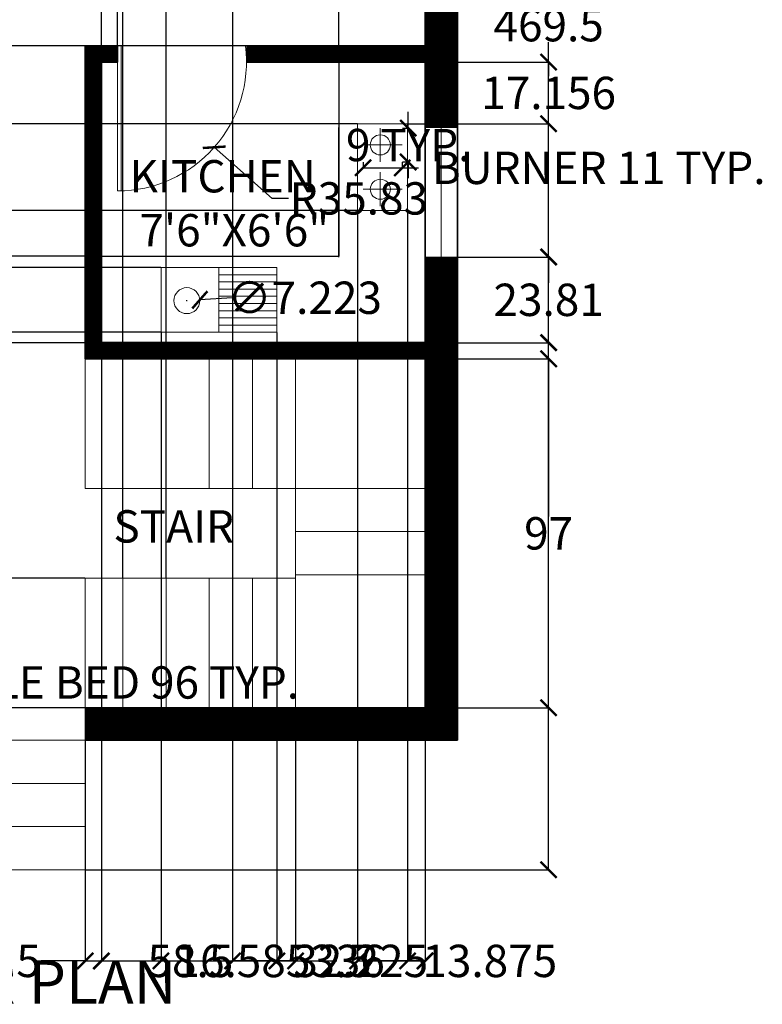
# Model space of a CAD drawing. Units: inches. Extents: x -1 to 426, y -6 to 532.
# Tile 2 of 4: x 219 to 426, y -6 to 267. Entities that reach past the tile are written whole.
import ezdxf

# ---------------------------------------------------------------- set-up
doc = ezdxf.new("R2010")
doc.units = ezdxf.units.IN
doc.header["$MEASUREMENT"] = 0
for name, color, linetype, lineweight in [('A-ANNO-DIMS', 2, 'Continuous', 18), ('A-ANNO-TEXT', 7, 'Continuous', 35), ('A-AREA-IDEN', 7, 'Continuous', 25), ('A-DOOR', 3, 'Continuous', 18), ('A-EQPM', 8, 'Continuous', 18), ('A-FLOR-CASE', 8, 'Continuous', 25), ('A-FLOR-FIXT', 8, 'Continuous', 18), ('A-FLOR-STRS', 42, 'Continuous', 18), ('A-GLAZ', 4, 'Continuous', 18)]:
    doc.layers.add(name, color=color, linetype=linetype, lineweight=lineweight)
doc.layers.add('A-WALL', color=159, linetype='Continuous', lineweight=35, true_color=0x223569)
doc.layers.add('A-WALL-PATT', color=177, linetype='Continuous', lineweight=13, true_color=0x2c4178)
doc.styles.get("Standard").update_dxf_attribs({"font": 'arial.ttf'})
doc.dimstyles.get("Standard").update_dxf_attribs({"dimtxt": 9, "dimasz": 4.5, "dimexe": 0.18, "dimexo": 0.0625, "dimgap": 0.09, "dimtad": 0, "dimtih": 1, "dimtoh": 1, "dimdec": 1, "dimzin": 0, "dimdsep": 46, "dimlunit": 4, "dimtxsty": 'Standard', "dimblk": 'ARCHTICK', "dimcen": 0.09, "dimadec": 0, "dimazin": 0, "dimtfac": 1, "dimtdec": 1, "dimtofl": 0, "dimtmove": 0, "dimatfit": 3, "dimfxl": 1, "dimtolj": 1, "dimtzin": 0, "dimarcsym": 0})

# ---------------------------------------------------------------- blocks, each defined once
blk = doc.blocks.new('WIN-36IN')
for p, q in [((0, 4.5), (36, 4.5)), ((0, -4.5), (0, 4.5)), ((36, 4.5), (36, -4.5)), ((0, 0), (36, 0)), ((36, -4.5), (0, -4.5))]:
    blk.add_line(p, q)
blk = doc.blocks.new('COOKTOP-BURNER')
for q in [(0, 4.66), (-4.8, 0), (6.12, 0), (0, -4.75)]:
    blk.add_line((0, 0), q)
blk.add_circle((0, 0), 2.79)
blk = doc.blocks.new('_ArchTick')
at = {"color": 0, "linetype": 'ByBlock', "const_width": 0.15}
blk.add_lwpolyline([(-0.5, -0.5), (0.5, 0.5)], dxfattribs=at)
blk = doc.blocks.new('*D11')
at = {"layer": 'A-ANNO-DIMS', "color": 0, "lineweight": -2, "transparency": 16777216}
for p, q in [((72.72, 97.36), (72.72, 82.85)), ((168.72, 97.36), (168.72, 82.85)), ((72.72, 83.03), (168.72, 83.03)), ((168.72, 83.03), (173.22, 83.03))]:
    blk.add_line(p, q, dxfattribs=at)
at = {"layer": 'Defpoints', "color": 0, "transparency": 16777216}
for p in [(72.72, 97.43), (168.72, 97.43), (168.72, 83.03)]:
    blk.add_point(p, dxfattribs=at)
at = {"layer": 'A-ANNO-DIMS', "color": 0, "lineweight": -2, "transparency": 16777216, "xscale": 4.5, "yscale": 4.5, "zscale": 4.5, "rotation": 180}
blk.add_blockref('_ArchTick', (72.72, 83.03), dxfattribs=at)
at = {"layer": 'A-ANNO-DIMS', "color": 0, "lineweight": -2, "transparency": 16777216, "xscale": 4.5, "yscale": 4.5, "zscale": 4.5}
blk.add_blockref('_ArchTick', (168.72, 83.03), dxfattribs=at)
at = {"layer": 'A-ANNO-DIMS', "color": 0, "transparency": 16777216, "insert": (237.26, 83.03), "char_height": 9, "attachment_point": 5}
blk.add_mtext('\\A1;DOUBLE BED 96 TYP.', dxfattribs=at)
blk = doc.blocks.new('*D15')
at = {"layer": 'A-ANNO-DIMS', "color": 0, "lineweight": -2, "transparency": 16777216}
for p, q in [((314.58, 227.64), (314.58, 225.89)), ((325.49, 227.64), (325.49, 225.89)), ((314.58, 226.07), (325.49, 226.07)), ((325.49, 226.07), (329.99, 226.07))]:
    blk.add_line(p, q, dxfattribs=at)
at = {"layer": 'Defpoints', "color": 0, "transparency": 16777216}
for p in [(314.58, 227.71), (325.49, 227.71), (325.49, 226.07)]:
    blk.add_point(p, dxfattribs=at)
at = {"layer": 'A-ANNO-DIMS', "color": 0, "lineweight": -2, "transparency": 16777216, "xscale": 4.5, "yscale": 4.5, "zscale": 4.5, "rotation": 180}
blk.add_blockref('_ArchTick', (314.58, 226.07), dxfattribs=at)
at = {"layer": 'A-ANNO-DIMS', "color": 0, "lineweight": -2, "transparency": 16777216, "xscale": 4.5, "yscale": 4.5, "zscale": 4.5}
blk.add_blockref('_ArchTick', (325.49, 226.07), dxfattribs=at)
at = {"layer": 'A-ANNO-DIMS', "color": 0, "transparency": 16777216, "insert": (380.08, 226.07), "char_height": 9, "attachment_point": 5}
blk.add_mtext('\\A1;BURNER 11 TYP.', dxfattribs=at)
blk = doc.blocks.new('*D16')
at = {"layer": 'A-ANNO-DIMS', "color": 0, "lineweight": -2, "transparency": 16777216}
for p, q in [((327.13, 237.11), (327.13, 241.61)), ((325.55, 237.11), (327.31, 237.11)), ((325.55, 227.71), (327.31, 227.71)), ((327.13, 227.71), (327.13, 223.21))]:
    blk.add_line(p, q, dxfattribs=at)
at = {"layer": 'Defpoints', "color": 0, "transparency": 16777216}
for p in [(325.49, 237.11), (327.13, 237.11), (325.49, 227.71)]:
    blk.add_point(p, dxfattribs=at)
at = {"layer": 'A-ANNO-DIMS', "color": 0, "lineweight": -2, "transparency": 16777216, "xscale": 4.5, "yscale": 4.5, "zscale": 4.5}
for p, rotation in [((327.13, 237.11), 270), ((327.13, 227.71), 90)]:
    blk.add_blockref('_ArchTick', p, dxfattribs=dict(at, rotation=rotation))
at = {"layer": 'A-ANNO-DIMS', "color": 0, "transparency": 16777216, "insert": (327.13, 232.41), "char_height": 9, "attachment_point": 5}
blk.add_mtext('\\A1;9 TYP.', dxfattribs=at)
blk = doc.blocks.new('*D18')
at = {"layer": 'A-ANNO-DIMS', "color": 0, "lineweight": -2, "transparency": 16777216}
for p, q in [((340.89, 500.48), (366.36, 500.48)), ((366.18, 500.48), (366.18, 270.42)), ((366.18, 30.98), (366.18, 261.05)), ((237.39, 30.98), (366.36, 30.98))]:
    blk.add_line(p, q, dxfattribs=at)
at = {"layer": 'Defpoints', "color": 0, "transparency": 16777216}
for p in [(340.82, 500.48), (366.18, 500.48), (237.32, 30.98)]:
    blk.add_point(p, dxfattribs=at)
at = {"layer": 'A-ANNO-DIMS', "color": 0, "lineweight": -2, "transparency": 16777216, "xscale": 4.5, "yscale": 4.5, "zscale": 4.5}
for p, rotation in [((366.18, 500.48), 90), ((366.18, 30.98), 270)]:
    blk.add_blockref('_ArchTick', p, dxfattribs=dict(at, rotation=rotation))
at = {"layer": 'A-ANNO-DIMS', "color": 0, "transparency": 16777216, "insert": (366.18, 265.73), "char_height": 9, "attachment_point": 5}
blk.add_mtext('\\A1;469.5', dxfattribs=at)
blk = doc.blocks.new('*D21')
at = {"layer": 'A-ANNO-DIMS', "color": 0, "lineweight": -2, "transparency": 16777216}
for p, q in [((188.82, 30.92), (188.82, 5.45)), ((237.32, 30.92), (237.32, 5.45)), ((188.82, 5.63), (201.08, 5.63)), ((237.32, 5.63), (225.07, 5.63))]:
    blk.add_line(p, q, dxfattribs=at)
at = {"layer": 'Defpoints', "color": 0, "transparency": 16777216}
for p in [(188.82, 30.98), (237.32, 30.98), (237.32, 5.63)]:
    blk.add_point(p, dxfattribs=at)
at = {"layer": 'A-ANNO-DIMS', "color": 0, "lineweight": -2, "transparency": 16777216, "xscale": 4.5, "yscale": 4.5, "zscale": 4.5, "rotation": 180}
blk.add_blockref('_ArchTick', (188.82, 5.63), dxfattribs=at)
at = {"layer": 'A-ANNO-DIMS', "color": 0, "lineweight": -2, "transparency": 16777216, "xscale": 4.5, "yscale": 4.5, "zscale": 4.5}
blk.add_blockref('_ArchTick', (237.32, 5.63), dxfattribs=at)
at = {"layer": 'A-ANNO-DIMS', "color": 0, "transparency": 16777216, "insert": (213.07, 5.63), "char_height": 9, "attachment_point": 5}
blk.add_mtext('\\A1;48.5', dxfattribs=at)
blk = doc.blocks.new('*D23')
at = {"layer": 'A-ANNO-DIMS', "color": 0, "lineweight": -2, "transparency": 16777216}
for p, q in [((278.32, 491.42), (278.32, 5.45)), ((331.82, 491.42), (331.82, 5.45)), ((278.32, 5.63), (293.26, 5.63)), ((331.82, 5.63), (316.89, 5.63))]:
    blk.add_line(p, q, dxfattribs=at)
at = {"layer": 'Defpoints', "color": 0, "transparency": 16777216}
for p in [(278.32, 491.48), (331.82, 491.48), (331.82, 5.63)]:
    blk.add_point(p, dxfattribs=at)
at = {"layer": 'A-ANNO-DIMS', "color": 0, "lineweight": -2, "transparency": 16777216, "xscale": 4.5, "yscale": 4.5, "zscale": 4.5, "rotation": 180}
blk.add_blockref('_ArchTick', (278.32, 5.63), dxfattribs=at)
at = {"layer": 'A-ANNO-DIMS', "color": 0, "lineweight": -2, "transparency": 16777216, "xscale": 4.5, "yscale": 4.5, "zscale": 4.5}
blk.add_blockref('_ArchTick', (331.82, 5.63), dxfattribs=at)
at = {"layer": 'A-ANNO-DIMS', "color": 0, "transparency": 16777216, "insert": (305.07, 5.63), "char_height": 9, "attachment_point": 5}
blk.add_mtext('\\A1;53.5', dxfattribs=at)
blk = doc.blocks.new('*D31')
at = {"layer": 'A-ANNO-DIMS', "color": 0, "lineweight": -2, "transparency": 16777216}
for p, q in [((331.89, 201.29), (366.36, 201.29)), ((366.18, 201.29), (366.18, 194.08)), ((366.18, 177.48), (366.18, 184.7)), ((331.89, 177.48), (366.36, 177.48))]:
    blk.add_line(p, q, dxfattribs=at)
at = {"layer": 'Defpoints', "color": 0, "transparency": 16777216}
for p in [(331.82, 201.29), (366.18, 201.29), (331.82, 177.48)]:
    blk.add_point(p, dxfattribs=at)
at = {"layer": 'A-ANNO-DIMS', "color": 0, "lineweight": -2, "transparency": 16777216, "xscale": 4.5, "yscale": 4.5, "zscale": 4.5}
for p, rotation in [((366.18, 201.29), 90), ((366.18, 177.48), 270)]:
    blk.add_blockref('_ArchTick', p, dxfattribs=dict(at, rotation=rotation))
at = {"layer": 'A-ANNO-DIMS', "color": 0, "transparency": 16777216, "insert": (366.18, 189.39), "char_height": 9, "attachment_point": 5}
blk.add_mtext('\\A1;23.81', dxfattribs=at)
blk = doc.blocks.new('*D32')
at = {"layer": 'A-ANNO-DIMS', "color": 0, "lineweight": -2, "transparency": 16777216}
for p, q in [((331.76, 293.06), (17.79, 293.06)), ((17.97, 293.06), (17.97, 281.21)), ((17.97, 259.98), (17.97, 271.83)), ((331.76, 259.98), (17.79, 259.98))]:
    blk.add_line(p, q, dxfattribs=at)
at = {"layer": 'Defpoints', "color": 0, "transparency": 16777216}
for p in [(17.97, 293.06), (331.82, 293.06), (331.82, 259.98)]:
    blk.add_point(p, dxfattribs=at)
at = {"layer": 'A-ANNO-DIMS', "color": 0, "lineweight": -2, "transparency": 16777216, "xscale": 4.5, "yscale": 4.5, "zscale": 4.5}
for p, rotation in [((17.97, 293.06), 90), ((17.97, 259.98), 270)]:
    blk.add_blockref('_ArchTick', p, dxfattribs=dict(at, rotation=rotation))
at = {"layer": 'A-ANNO-DIMS', "color": 0, "transparency": 16777216, "insert": (17.97, 276.52), "char_height": 9, "attachment_point": 5}
blk.add_mtext('\\A1;33.08', dxfattribs=at)
blk = doc.blocks.new('*D34')
at = {"layer": 'A-ANNO-DIMS', "color": 0, "lineweight": -2, "transparency": 16777216}
for p, q in [((237.26, 111.98), (17.79, 111.98)), ((17.97, 111.98), (17.97, 98.67)), ((17.97, 75.98), (17.97, 89.29)), ((237.26, 75.98), (17.79, 75.98))]:
    blk.add_line(p, q, dxfattribs=at)
at = {"layer": 'Defpoints', "color": 0, "transparency": 16777216}
for p in [(17.97, 111.98), (237.32, 111.98), (237.32, 75.98)]:
    blk.add_point(p, dxfattribs=at)
at = {"layer": 'A-ANNO-DIMS', "color": 0, "lineweight": -2, "transparency": 16777216, "xscale": 4.5, "yscale": 4.5, "zscale": 4.5}
for p, rotation in [((17.97, 111.98), 90), ((17.97, 75.98), 270)]:
    blk.add_blockref('_ArchTick', p, dxfattribs=dict(at, rotation=rotation))
at = {"layer": 'A-ANNO-DIMS', "color": 0, "transparency": 16777216, "insert": (17.97, 93.98), "char_height": 9, "attachment_point": 5}
blk.add_mtext('\\A1;36', dxfattribs=at)
blk = doc.blocks.new('*D35')
at = {"layer": 'A-ANNO-DIMS', "color": 0, "lineweight": -2, "transparency": 16777216}
for p, q in [((247.82, 112.04), (247.82, 526.02)), ((247.82, 525.84), (259.82, 525.84)), ((259.82, 112.04), (259.82, 526.02)), ((259.82, 525.84), (264.32, 525.84))]:
    blk.add_line(p, q, dxfattribs=at)
at = {"layer": 'Defpoints', "color": 0, "transparency": 16777216}
for p in [(259.82, 525.84), (247.82, 111.98), (259.82, 111.98)]:
    blk.add_point(p, dxfattribs=at)
at = {"layer": 'A-ANNO-DIMS', "color": 0, "lineweight": -2, "transparency": 16777216, "xscale": 4.5, "yscale": 4.5, "zscale": 4.5, "rotation": 180}
blk.add_blockref('_ArchTick', (247.82, 525.84), dxfattribs=at)
at = {"layer": 'A-ANNO-DIMS', "color": 0, "lineweight": -2, "transparency": 16777216, "xscale": 4.5, "yscale": 4.5, "zscale": 4.5}
blk.add_blockref('_ArchTick', (259.82, 525.84), dxfattribs=at)
at = {"layer": 'A-ANNO-DIMS', "color": 0, "transparency": 16777216, "insert": (270.39, 525.84), "char_height": 9, "attachment_point": 5}
blk.add_mtext('\\A1;12', dxfattribs=at)
blk = doc.blocks.new('*D36')
at = {"layer": 'A-ANNO-DIMS', "color": 0, "lineweight": -2, "transparency": 16777216}
for p, q in [((258.4, 180.34), (258.4, 5.45)), ((290.63, 180.34), (290.63, 5.45)), ((258.4, 5.63), (290.63, 5.63)), ((290.63, 5.63), (295.13, 5.63))]:
    blk.add_line(p, q, dxfattribs=at)
at = {"layer": 'Defpoints', "color": 0, "transparency": 16777216}
for p in [(258.4, 180.4), (290.63, 180.4), (290.63, 5.63)]:
    blk.add_point(p, dxfattribs=at)
at = {"layer": 'A-ANNO-DIMS', "color": 0, "lineweight": -2, "transparency": 16777216, "xscale": 4.5, "yscale": 4.5, "zscale": 4.5, "rotation": 180}
blk.add_blockref('_ArchTick', (258.4, 5.63), dxfattribs=at)
at = {"layer": 'A-ANNO-DIMS', "color": 0, "lineweight": -2, "transparency": 16777216, "xscale": 4.5, "yscale": 4.5, "zscale": 4.5}
blk.add_blockref('_ArchTick', (290.63, 5.63), dxfattribs=at)
at = {"layer": 'A-ANNO-DIMS', "color": 0, "transparency": 16777216, "insert": (313.93, 5.63), "char_height": 9, "attachment_point": 5}
blk.add_mtext('\\A1;32.225', dxfattribs=at)
blk = doc.blocks.new('*D37')
at = {"layer": 'A-ANNO-DIMS', "color": 0, "lineweight": -2, "transparency": 16777216}
for p, q in [((258.34, 198.36), (17.79, 198.36)), ((17.97, 198.36), (17.97, 194.07)), ((17.97, 180.4), (17.97, 184.7)), ((258.34, 180.4), (17.79, 180.4))]:
    blk.add_line(p, q, dxfattribs=at)
at = {"layer": 'Defpoints', "color": 0, "transparency": 16777216}
for p in [(17.97, 198.36), (258.4, 198.36), (258.4, 180.4)]:
    blk.add_point(p, dxfattribs=at)
at = {"layer": 'A-ANNO-DIMS', "color": 0, "lineweight": -2, "transparency": 16777216, "xscale": 4.5, "yscale": 4.5, "zscale": 4.5}
for p, rotation in [((17.97, 198.36), 90), ((17.97, 180.4), 270)]:
    blk.add_blockref('_ArchTick', p, dxfattribs=dict(at, rotation=rotation))
at = {"layer": 'A-ANNO-DIMS', "color": 0, "transparency": 16777216, "insert": (17.97, 189.38), "char_height": 9, "attachment_point": 5}
blk.add_mtext('\\A1;17.96', dxfattribs=at)
blk = doc.blocks.new('*D38')
at = {"layer": 'A-ANNO-DIMS', "color": 0, "lineweight": -2, "transparency": 16777216}
for p, q in [((307.82, 255.54), (307.82, 526.02)), ((307.82, 525.84), (313.23, 525.84)), ((331.82, 525.84), (326.42, 525.84)), ((331.82, 255.54), (331.82, 526.02))]:
    blk.add_line(p, q, dxfattribs=at)
at = {"layer": 'Defpoints', "color": 0, "transparency": 16777216}
for p in [(331.82, 525.84), (307.82, 255.48), (331.82, 255.48)]:
    blk.add_point(p, dxfattribs=at)
at = {"layer": 'A-ANNO-DIMS', "color": 0, "lineweight": -2, "transparency": 16777216, "xscale": 4.5, "yscale": 4.5, "zscale": 4.5, "rotation": 180}
blk.add_blockref('_ArchTick', (307.82, 525.84), dxfattribs=at)
at = {"layer": 'A-ANNO-DIMS', "color": 0, "lineweight": -2, "transparency": 16777216, "xscale": 4.5, "yscale": 4.5, "zscale": 4.5}
blk.add_blockref('_ArchTick', (331.82, 525.84), dxfattribs=at)
at = {"layer": 'A-ANNO-DIMS', "color": 0, "transparency": 16777216, "insert": (319.82, 525.84), "char_height": 9, "attachment_point": 5}
blk.add_mtext('\\A1;24', dxfattribs=at)
blk = doc.blocks.new('*D42')
at = {"layer": 'A-ANNO-DIMS', "color": 0, "lineweight": -2, "transparency": 16777216}
for p, q in [((331.89, 172.98), (366.36, 172.98)), ((366.18, 172.98), (366.18, 129.17)), ((366.18, 75.98), (366.18, 119.8)), ((331.89, 75.98), (366.36, 75.98))]:
    blk.add_line(p, q, dxfattribs=at)
at = {"layer": 'Defpoints', "color": 0, "transparency": 16777216}
for p in [(331.82, 172.98), (366.18, 172.98), (331.82, 75.98)]:
    blk.add_point(p, dxfattribs=at)
at = {"layer": 'A-ANNO-DIMS', "color": 0, "lineweight": -2, "transparency": 16777216, "xscale": 4.5, "yscale": 4.5, "zscale": 4.5}
for p, rotation in [((366.18, 172.98), 90), ((366.18, 75.98), 270)]:
    blk.add_blockref('_ArchTick', p, dxfattribs=dict(at, rotation=rotation))
at = {"layer": 'A-ANNO-DIMS', "color": 0, "transparency": 16777216, "insert": (366.18, 124.48), "char_height": 9, "attachment_point": 5}
blk.add_mtext('\\A1;97', dxfattribs=at)
blk = doc.blocks.new('*D43')
at = {"layer": 'A-ANNO-DIMS', "color": 0, "lineweight": -2, "transparency": 16777216}
for p, q in [((295.82, 75.92), (295.82, 5.45)), ((331.82, 75.92), (331.82, 5.45)), ((295.82, 5.63), (307.29, 5.63)), ((331.82, 5.63), (320.35, 5.63))]:
    blk.add_line(p, q, dxfattribs=at)
at = {"layer": 'Defpoints', "color": 0, "transparency": 16777216}
for p in [(295.82, 75.98), (331.82, 75.98), (331.82, 5.63)]:
    blk.add_point(p, dxfattribs=at)
at = {"layer": 'A-ANNO-DIMS', "color": 0, "lineweight": -2, "transparency": 16777216, "xscale": 4.5, "yscale": 4.5, "zscale": 4.5, "rotation": 180}
blk.add_blockref('_ArchTick', (295.82, 5.63), dxfattribs=at)
at = {"layer": 'A-ANNO-DIMS', "color": 0, "lineweight": -2, "transparency": 16777216, "xscale": 4.5, "yscale": 4.5, "zscale": 4.5}
blk.add_blockref('_ArchTick', (331.82, 5.63), dxfattribs=at)
at = {"layer": 'A-ANNO-DIMS', "color": 0, "transparency": 16777216, "insert": (313.82, 5.63), "char_height": 9, "attachment_point": 5}
blk.add_mtext('\\A1;36', dxfattribs=at)
blk = doc.blocks.new('*D44')
at = {"layer": 'A-ANNO-DIMS', "color": 0, "lineweight": -2, "transparency": 16777216}
for p, q in [((237.32, 75.92), (237.32, 5.45)), ((295.82, 75.92), (295.82, 5.45)), ((237.32, 5.63), (254.76, 5.63)), ((295.82, 5.63), (278.39, 5.63))]:
    blk.add_line(p, q, dxfattribs=at)
at = {"layer": 'Defpoints', "color": 0, "transparency": 16777216}
for p in [(237.32, 75.98), (295.82, 75.98), (295.82, 5.63)]:
    blk.add_point(p, dxfattribs=at)
at = {"layer": 'A-ANNO-DIMS', "color": 0, "lineweight": -2, "transparency": 16777216, "xscale": 4.5, "yscale": 4.5, "zscale": 4.5, "rotation": 180}
blk.add_blockref('_ArchTick', (237.32, 5.63), dxfattribs=at)
at = {"layer": 'A-ANNO-DIMS', "color": 0, "lineweight": -2, "transparency": 16777216, "xscale": 4.5, "yscale": 4.5, "zscale": 4.5}
blk.add_blockref('_ArchTick', (295.82, 5.63), dxfattribs=at)
at = {"layer": 'A-ANNO-DIMS', "color": 0, "transparency": 16777216, "insert": (266.57, 5.63), "char_height": 9, "attachment_point": 5}
blk.add_mtext('\\A1;58.5', dxfattribs=at)
blk = doc.blocks.new('*D45')
at = {"layer": 'A-ANNO-DIMS', "color": 0, "lineweight": -2, "transparency": 16777216}
for p, q in [((241.76, 201.48), (17.79, 201.48)), ((17.97, 201.48), (17.97, 194.09)), ((17.97, 177.48), (17.97, 184.87)), ((241.76, 177.48), (17.79, 177.48))]:
    blk.add_line(p, q, dxfattribs=at)
at = {"layer": 'Defpoints', "color": 0, "transparency": 16777216}
for p in [(17.97, 201.48), (241.82, 201.48), (241.82, 177.48)]:
    blk.add_point(p, dxfattribs=at)
at = {"layer": 'A-ANNO-DIMS', "color": 0, "lineweight": -2, "transparency": 16777216, "xscale": 4.5, "yscale": 4.5, "zscale": 4.5}
for p, rotation in [((17.97, 201.48), 90), ((17.97, 177.48), 270)]:
    blk.add_blockref('_ArchTick', p, dxfattribs=dict(at, rotation=rotation))
at = {"layer": 'A-ANNO-DIMS', "color": 0, "transparency": 16777216, "insert": (17.97, 189.48), "char_height": 9, "attachment_point": 5}
blk.add_mtext('\\A1;24', dxfattribs=at)
blk = doc.blocks.new('*D46')
at = {"layer": 'A-ANNO-DIMS', "color": 0, "lineweight": -2, "transparency": 16777216}
for p, q in [((241.82, 255.54), (241.82, 526.02)), ((241.82, 525.84), (246.32, 525.84)), ((246.32, 255.54), (246.32, 526.02)), ((246.32, 525.84), (250.82, 525.84))]:
    blk.add_line(p, q, dxfattribs=at)
at = {"layer": 'Defpoints', "color": 0, "transparency": 16777216}
for p in [(246.32, 525.84), (241.82, 255.48), (246.32, 255.48)]:
    blk.add_point(p, dxfattribs=at)
at = {"layer": 'A-ANNO-DIMS', "color": 0, "lineweight": -2, "transparency": 16777216, "xscale": 4.5, "yscale": 4.5, "zscale": 4.5, "rotation": 180}
blk.add_blockref('_ArchTick', (241.82, 525.84), dxfattribs=at)
at = {"layer": 'A-ANNO-DIMS', "color": 0, "lineweight": -2, "transparency": 16777216, "xscale": 4.5, "yscale": 4.5, "zscale": 4.5}
blk.add_blockref('_ArchTick', (246.32, 525.84), dxfattribs=at)
at = {"layer": 'A-ANNO-DIMS', "color": 0, "transparency": 16777216, "insert": (259.32, 525.84), "char_height": 9, "attachment_point": 5}
blk.add_mtext('\\A1;4.5', dxfattribs=at)
blk = doc.blocks.new('*D48')
at = {"layer": 'A-ANNO-DIMS', "color": 0, "lineweight": -2, "transparency": 16777216}
for p, q in [((258.4, 180.34), (258.4, 5.45)), ((241.82, 177.42), (241.82, 5.45)), ((241.82, 5.63), (258.4, 5.63)), ((258.4, 5.63), (262.9, 5.63))]:
    blk.add_line(p, q, dxfattribs=at)
at = {"layer": 'Defpoints', "color": 0, "transparency": 16777216}
for p in [(258.4, 180.4), (241.82, 177.48), (258.4, 5.63)]:
    blk.add_point(p, dxfattribs=at)
at = {"layer": 'A-ANNO-DIMS', "color": 0, "lineweight": -2, "transparency": 16777216, "xscale": 4.5, "yscale": 4.5, "zscale": 4.5, "rotation": 180}
blk.add_blockref('_ArchTick', (241.82, 5.63), dxfattribs=at)
at = {"layer": 'A-ANNO-DIMS', "color": 0, "lineweight": -2, "transparency": 16777216, "xscale": 4.5, "yscale": 4.5, "zscale": 4.5}
blk.add_blockref('_ArchTick', (258.4, 5.63), dxfattribs=at)
at = {"layer": 'A-ANNO-DIMS', "color": 0, "transparency": 16777216, "insert": (277.76, 5.63), "char_height": 9, "attachment_point": 5}
blk.add_mtext('\\A1;16.58', dxfattribs=at)
blk = doc.blocks.new('*D49')
at = {"layer": 'A-ANNO-DIMS', "color": 0, "lineweight": -2, "transparency": 16777216}
for p, q in [((331.89, 255.48), (366.36, 255.48)), ((366.18, 255.48), (366.18, 251.59)), ((366.18, 238.33), (366.18, 242.22)), ((327, 238.33), (366.36, 238.33))]:
    blk.add_line(p, q, dxfattribs=at)
at = {"layer": 'Defpoints', "color": 0, "transparency": 16777216}
for p in [(331.82, 255.48), (366.18, 255.48), (326.94, 238.33)]:
    blk.add_point(p, dxfattribs=at)
at = {"layer": 'A-ANNO-DIMS', "color": 0, "lineweight": -2, "transparency": 16777216, "xscale": 4.5, "yscale": 4.5, "zscale": 4.5}
for p, rotation in [((366.18, 255.48), 90), ((366.18, 238.33), 270)]:
    blk.add_blockref('_ArchTick', p, dxfattribs=dict(at, rotation=rotation))
at = {"layer": 'A-ANNO-DIMS', "color": 0, "transparency": 16777216, "insert": (366.18, 246.9), "char_height": 9, "attachment_point": 5}
blk.add_mtext('\\A1;17.156', dxfattribs=at)
blk = doc.blocks.new('*D52')
at = {"layer": 'A-ANNO-DIMS', "color": 0, "lineweight": -2, "transparency": 16777216}
for p, q in [((313.06, 214.18), (313.06, 5.45)), ((326.94, 214.18), (326.94, 5.45)), ((313.06, 5.63), (326.94, 5.63)), ((326.94, 5.63), (331.44, 5.63))]:
    blk.add_line(p, q, dxfattribs=at)
at = {"layer": 'Defpoints', "color": 0, "transparency": 16777216}
for p in [(313.06, 214.24), (326.94, 214.24), (326.94, 5.63)]:
    blk.add_point(p, dxfattribs=at)
at = {"layer": 'A-ANNO-DIMS', "color": 0, "lineweight": -2, "transparency": 16777216, "xscale": 4.5, "yscale": 4.5, "zscale": 4.5, "rotation": 180}
blk.add_blockref('_ArchTick', (313.06, 5.63), dxfattribs=at)
at = {"layer": 'A-ANNO-DIMS', "color": 0, "lineweight": -2, "transparency": 16777216, "xscale": 4.5, "yscale": 4.5, "zscale": 4.5}
blk.add_blockref('_ArchTick', (326.94, 5.63), dxfattribs=at)
at = {"layer": 'A-ANNO-DIMS', "color": 0, "transparency": 16777216, "insert": (349.82, 5.63), "char_height": 9, "attachment_point": 5}
blk.add_mtext('\\A1;13.875', dxfattribs=at)
blk = doc.blocks.new('*D53')
at = {"layer": 'A-ANNO-DIMS', "color": 0, "lineweight": -2, "transparency": 16777216}
for p, q in [((313, 238.33), (17.79, 238.33)), ((17.97, 238.33), (17.97, 230.97)), ((17.97, 214.24), (17.97, 221.6)), ((313, 214.24), (17.79, 214.24))]:
    blk.add_line(p, q, dxfattribs=at)
at = {"layer": 'Defpoints', "color": 0, "transparency": 16777216}
for p in [(17.97, 238.33), (313.06, 238.33), (313.06, 214.24)]:
    blk.add_point(p, dxfattribs=at)
at = {"layer": 'A-ANNO-DIMS', "color": 0, "lineweight": -2, "transparency": 16777216, "xscale": 4.5, "yscale": 4.5, "zscale": 4.5}
for p, rotation in [((17.97, 238.33), 90), ((17.97, 214.24), 270)]:
    blk.add_blockref('_ArchTick', p, dxfattribs=dict(at, rotation=rotation))
at = {"layer": 'A-ANNO-DIMS', "color": 0, "transparency": 16777216, "insert": (17.97, 226.28), "char_height": 9, "attachment_point": 5}
blk.add_mtext('\\A1;24.087', dxfattribs=at)
blk = doc.blocks.new('*D56')
at = {"layer": 'A-ANNO-DIMS', "color": 0, "lineweight": -2, "transparency": 16777216}
for p, q in [((246.23, 255.48), (246.41, 255.48)), ((246.32, 255.39), (246.32, 255.57)), ((289.33, 217.58), (273.2, 231.79)), ((293.83, 217.58), (289.33, 217.58))]:
    blk.add_line(p, q, dxfattribs=at)
at = {"layer": 'Defpoints', "color": 0, "transparency": 16777216}
for p in [(246.32, 255.48), (273.2, 231.79)]:
    blk.add_point(p, dxfattribs=at)
at = {"layer": 'A-ANNO-DIMS', "color": 0, "lineweight": -2, "transparency": 16777216, "xscale": 4.5, "yscale": 4.5, "zscale": 4.5, "rotation": 138.6071113163995}
blk.add_blockref('_ArchTick', (273.2, 231.79), dxfattribs=at)
at = {"layer": 'A-ANNO-DIMS', "color": 0, "transparency": 16777216, "insert": (313.41, 217.58), "char_height": 9, "attachment_point": 5}
blk.add_mtext('\\A1;R35.83', dxfattribs=at)
blk = doc.blocks.new('*D58')
at = {"layer": 'A-ANNO-DIMS', "color": 0, "lineweight": -2, "transparency": 16777216}
for p, q in [((265.5, 189.16), (265.68, 189.16)), ((265.59, 189.07), (265.59, 189.25)), ((278.18, 189.97), (269.2, 189.39))]:
    blk.add_line(p, q, dxfattribs=at)
at = {"layer": 'Defpoints', "color": 0, "transparency": 16777216}
for p in [(261.99, 188.93), (269.2, 189.39)]:
    blk.add_point(p, dxfattribs=at)
at = {"layer": 'A-ANNO-DIMS', "color": 0, "lineweight": -2, "transparency": 16777216, "xscale": 4.5, "yscale": 4.5, "zscale": 4.5, "rotation": 183.6720781902935}
blk.add_blockref('_ArchTick', (269.2, 189.39), dxfattribs=at)
at = {"layer": 'A-ANNO-DIMS', "color": 0, "transparency": 16777216, "insert": (298.35, 189.97), "char_height": 9, "attachment_point": 5}
blk.add_mtext('\\A1;∅7.223', dxfattribs=at)

msp = doc.modelspace()

# ---------------------------------------------------------------- hatches: boundary and pattern name
at = {"layer": 'A-WALL-PATT'}
h = msp.add_hatch(dxfattribs=at)
h.set_pattern_fill('ANSI31', color=256)
h.set_pattern_definition([(45, (-574.8435, 0), (-0.088388348, 0.088388348), [])])
h.paths.add_polyline_path([(100.3238, 500.4824), (43.3238, 500.4824), (43.3238, 452.5693), (52.3238, 452.5693), (52.3238, 491.4824), (100.3238, 491.4824)])
h.paths.add_polyline_path([(242.3238, 500.4824), (136.3238, 500.4824), (136.3238, 491.4824), (184.3238, 491.4824), (184.3238, 407.9824), (188.8238, 407.9824), (193.3238, 407.9824), (193.3238, 412.4824), (188.8238, 412.4824), (188.8238, 491.4824), (242.3238, 491.4824)])
h.paths.add_polyline_path([(340.8238, 500.4824), (278.3238, 500.4824), (278.3238, 491.4824), (331.8238, 491.4824), (331.8238, 478.8941), (340.8238, 478.8941)])
h.paths.add_polyline_path([(331.8238, 412.4824), (229.3238, 412.4824), (229.3238, 407.9824), (331.8238, 407.9824)])
h.paths.add_polyline_path([(340.8238, 430.8941), (331.8238, 430.8941), (331.8238, 341.0593), (340.8238, 341.0593)])
h.paths.add_polyline_path([(340.8238, 293.0593), (331.8238, 293.0593), (331.8238, 259.9824), (282.3238, 259.9824), (282.3238, 255.4824), (331.8238, 255.4824), (331.8238, 237.2917), (340.8238, 237.2917)])
h.paths.add_polyline_path([(340.8238, 153.5275), (340.8238, 201.2917), (331.8238, 201.2917), (331.8238, 177.4824), (241.8238, 177.4824), (241.8238, 255.4824), (246.3238, 255.4824), (246.3238, 259.9824), (237.3238, 259.9824), (237.3238, 255.4824), (237.3238, 172.9824), (331.8238, 172.9824), (331.8238, 153.5275), (331.8238, 75.9824), (237.3238, 75.9824), (237.3238, 66.9824), (340.8238, 66.9824)])
h.paths.add_polyline_path([(98.5766, 75.9824), (52.3238, 75.9824), (52.3238, 138.3606), (43.3238, 138.3606), (43.3238, 66.9824), (52.3238, 66.9824), (98.5766, 66.9824)])
h.paths.add_polyline_path([(188.8238, 75.9824), (188.8238, 153.5275), (188.8238, 209.4042, -0.02664097), (184.3238, 209.1642), (184.3238, 153.5275), (184.3238, 75.9824), (136.8238, 75.9824), (134.5766, 75.9824), (134.5766, 66.9824), (136.8238, 66.9824), (188.8238, 66.9824)])
h.paths.add_polyline_path([(52.3238, 255.9824), (96.3583, 255.9824), (96.3583, 260.4824), (52.3238, 260.4824), (52.3238, 272.4986), (43.3238, 272.4986), (43.3238, 186.3606), (52.3238, 186.3606)])
h.paths.add_polyline_path([(52.3238, 404.5693), (43.3238, 404.5693), (43.3238, 349.9808), (52.3238, 349.9808), (52.3238, 360.9824), (184.3238, 360.9824), (184.3238, 312.9824), (173.036, 312.9824), (173.036, 308.4824), (184.3238, 308.4824), (188.8238, 308.4824), (188.8238, 365.4824), (184.3238, 365.4824), (52.3238, 365.4824)])
h.paths.add_polyline_path([(188.8238, 260.4824), (136.8238, 260.4824), (136.8238, 308.4824), (136.8238, 312.9824), (52.3238, 312.9824), (52.3238, 332.4824), (43.3238, 332.4824), (43.3238, 308.4824), (43.3238, 296.4986), (52.3238, 296.4986), (52.3238, 298.8674), (52.3238, 308.4824), (132.3238, 308.4824), (132.3238, 260.4824), (132.3238, 255.9824), (136.8238, 255.9824), (184.3238, 255.9824), (184.3238, 251.4824), (186.5738, 251.4824), (188.8238, 251.4824), (188.8238, 255.9824)])

# ---------------------------------------------------------------- linework, layer by layer
at = {"layer": 'A-DOOR'}
for p, q in [((246.3238, 259.9824), (282.3238, 259.9824)), ((246.3238, 259.9824), (246.3238, 219.6537)), ((247.3238, 259.9824), (247.3238, 219.6677))]:
    msp.add_line(p, q, dxfattribs=at)
msp.add_arc((246.3238, 255.4824), 35.8287, 270, 7.215276, dxfattribs=at)
at = {"layer": 'A-EQPM'}
for p, q in [((313.0636, 238.326), (326.9391, 238.326)), ((313.0636, 214.2386), (313.0636, 238.326)), ((326.9391, 238.326), (326.9391, 214.2386)), ((326.9391, 214.2386), (313.0636, 214.2386))]:
    msp.add_line(p, q, dxfattribs=at)
at = {"layer": 'A-FLOR-CASE'}
for p, q in [((307.8238, 255.4824), (307.8238, 201.4824)), ((307.8238, 201.2917), (307.8238, 237.2917)), ((241.8238, 201.4824), (307.8238, 201.4824))]:
    msp.add_line(p, q, dxfattribs=at)
at = {"layer": 'A-FLOR-FIXT'}
for p, q in [((258.4022, 198.3607), (290.6274, 198.3607)), ((258.4022, 180.4022), (258.4022, 198.3607)), ((274.5148, 180.4022), (274.5148, 198.3607)), ((290.6274, 198.3607), (290.6274, 180.4022)), ((274.5148, 196.3607), (290.6274, 196.3607)), ((274.5148, 194.3607), (290.6274, 194.3607)), ((274.5148, 192.3607), (290.6274, 192.3607)), ((274.5148, 190.3607), (290.6274, 190.3607)), ((274.5148, 188.3607), (290.6274, 188.3607)), ((274.5148, 188.3607), (290.6274, 188.3607)), ((274.5148, 186.3607), (290.6274, 186.3607)), ((274.5148, 184.3607), (290.6274, 184.3607)), ((274.5148, 182.3607), (290.6274, 182.3607)), ((290.6274, 180.4022), (258.4022, 180.4022))]:
    msp.add_line(p, q, dxfattribs=at)
msp.add_circle((265.591, 189.1612), 3.6117, dxfattribs=at)
at = {"layer": 'A-FLOR-STRS'}
for p, q in [((237.3238, 172.9824), (237.3238, 136.9824)), ((247.8238, 136.9824), (247.8238, 172.9824)), ((259.8238, 136.9824), (259.8238, 172.9824)), ((271.8238, 136.9824), (271.8238, 172.9824)), ((283.8238, 136.9824), (283.8238, 172.9824)), ((295.8238, 136.9824), (295.8238, 172.9824)), ((237.3238, 136.9824), (295.8238, 136.9824)), ((295.8238, 136.9824), (295.8238, 111.9824)), ((295.8238, 136.9824), (331.8238, 136.9824)), ((295.8238, 124.9824), (331.8238, 124.9824)), ((295.8238, 112.9824), (331.8238, 112.9824)), ((237.3238, 111.9824), (295.8238, 111.9824)), ((237.3238, 111.9824), (237.3238, 66.9824)), ((247.8238, 111.9824), (247.8238, 75.9824)), ((259.8238, 111.9824), (259.8238, 75.9824)), ((271.8238, 111.9824), (271.8238, 75.9824)), ((283.8238, 111.9824), (283.8238, 75.9824)), ((295.8238, 111.9824), (295.8238, 75.9824)), ((237.3238, 66.9824), (188.8238, 66.9824)), ((237.3238, 30.9824), (237.3238, 66.9824)), ((237.3238, 54.9824), (188.8238, 54.9824)), ((237.3238, 42.9824), (188.8238, 42.9824)), ((237.3238, 30.9824), (188.8238, 30.9824))]:
    msp.add_line(p, q, dxfattribs=at)
at = {"layer": 'A-WALL'}
for p, q in [((340.8238, 500.4824), (340.8238, 153.5275)), ((331.8238, 491.4824), (331.8238, 259.9824)), ((237.3238, 259.9824), (246.3238, 259.9824)), ((237.3238, 255.4824), (237.3238, 259.9824)), ((246.3238, 255.4824), (246.3238, 259.9824)), ((282.3238, 255.4824), (282.3238, 259.9824)), ((282.3238, 259.9824), (331.8238, 259.9824)), ((237.3238, 255.4824), (237.3238, 172.9824)), ((241.8238, 255.4824), (246.3238, 255.4824)), ((241.8238, 255.4824), (241.8238, 177.4824)), ((282.3238, 255.4824), (331.8238, 255.4824)), ((331.8238, 255.4824), (331.8238, 177.4824)), ((241.8238, 177.4824), (331.8238, 177.4824)), ((237.3238, 172.9824), (331.8238, 172.9824)), ((331.8238, 172.9824), (331.8238, 153.5275)), ((331.8238, 153.5275), (331.8238, 75.9824)), ((340.8238, 153.5275), (340.8238, 66.9824)), ((237.3238, 75.9824), (331.8238, 75.9824)), ((237.3238, 66.9824), (340.8238, 66.9824))]:
    msp.add_line(p, q, dxfattribs=at)

# ---------------------------------------------------------------- block references
at = {"layer": 'A-EQPM'}
msp.add_blockref('COOKTOP-BURNER', (319.3764, 232.4507), dxfattribs=at)
at = {"layer": 'A-EQPM', "extrusion": (0, 0, -1), "zscale": -1, "rotation": 180}
msp.add_blockref('COOKTOP-BURNER', (-319.3764, 220.1139), dxfattribs=at)
at = {"layer": 'A-GLAZ', "rotation": 270}
msp.add_blockref('WIN-36IN', (336.3238, 237.2917), dxfattribs=at)

# ---------------------------------------------------------------- texts
at = {"layer": 'A-ANNO-TEXT', "insert": (85.5965, 5.7797), "char_height": 12, "attachment_point": 1}
msp.add_mtext_dynamic_manual_height_columns('  GROUND FLOOR PLAN', width=229.541527, gutter_width=1, heights=[0], dxfattribs=at)
at = {"layer": 'A-AREA-IDEN', "char_height": 9, "attachment_point": 1}
for s, insert in [(' KITCHEN\\P  7\'6"X6\'6"', (246.8874, 228.2374)), ('   STAIR', (236.9183, 130.9154))]:
    msp.add_mtext_dynamic_manual_height_columns(s, width=229.541527, gutter_width=1, heights=[0], dxfattribs=dict(at, insert=insert))

# ---------------------------------------------------------------- dimensions: what is measured, and where the dimension line sits
at = {"layer": 'A-ANNO-DIMS'}
for base, p1, p2, override, picture, middle in [((246.3238, 525.8389), (241.8238, 255.4824), (246.3238, 255.4824), {"dimdec": 1, "dimlfac": 1, "dimrnd": 0, "dimzin": 0, "dimdsep": 46, "dimlunit": 2}, '*D46', (259.3214, 525.8389)), ((259.8238, 525.8389), (247.8238, 111.9824), (259.8238, 111.9824), {"dimdec": 0, "dimlfac": 1, "dimrnd": 0, "dimzin": 0, "dimdsep": 46, "dimlunit": 2}, '*D35', (270.3902, 525.8389)), ((331.8238, 525.8389), (307.8238, 255.4824), (331.8238, 255.4824), {"dimdec": 0, "dimlfac": 1, "dimrnd": 0, "dimzin": 0, "dimdsep": 46, "dimlunit": 2}, '*D38', (319.8238, 525.8389)), ((331.8238, 5.6259), (278.3238, 491.4824), (331.8238, 491.4824), {"dimdec": 1, "dimlfac": 1, "dimrnd": 0, "dimzin": 0, "dimdsep": 46, "dimlunit": 2}, '*D23', (305.0738, 5.6259)), ((326.939098, 5.625908), (313.063605, 214.238595), (326.939098, 214.238595), {"dimdec": 3, "dimlfac": 1, "dimrnd": 0, "dimzin": 0, "dimdsep": 46, "dimlunit": 2}, '*D52', (349.820708, 5.625908)), ((258.4022, 5.6259), (241.8238, 177.4824), (258.4022, 180.4022), {"dimdec": 2, "dimlfac": 1, "dimrnd": 0, "dimzin": 0, "dimdsep": 46, "dimlunit": 2}, '*D48', (277.763, 5.6259)), ((290.6274, 5.6259), (258.4022, 180.4022), (290.6274, 180.4022), {"dimdec": 3, "dimlfac": 1, "dimrnd": 0, "dimzin": 0, "dimdsep": 46, "dimlunit": 2}, '*D36', (313.9295, 5.6259)), ((295.8238, 5.6259), (237.3238, 75.9824), (295.8238, 75.9824), {"dimdec": 1, "dimlfac": 1, "dimrnd": 0, "dimzin": 0, "dimdsep": 46, "dimlunit": 2}, '*D44', (266.5738, 5.6259)), ((331.8238, 5.6259), (295.8238, 75.9824), (331.8238, 75.9824), {"dimdec": 0, "dimlfac": 1, "dimrnd": 0, "dimzin": 0, "dimdsep": 46, "dimlunit": 2}, '*D43', (313.8238, 5.6259)), ((237.3238, 5.6259), (188.8238, 30.9824), (237.3238, 30.9824), {"dimdec": 1, "dimlfac": 1, "dimrnd": 0, "dimzin": 0, "dimdsep": 46, "dimlunit": 2}, '*D21', (213.0738, 5.6259))]:
    dim = msp.add_linear_dim(base=base, p1=p1, p2=p2, dimstyle='Standard', override=override, dxfattribs=at)
    dim.commit()
    dim.dimension.update_dxf_attribs({"geometry": picture, "text_midpoint": middle})
for base, p1, p2, override, picture, middle in [((366.1803, 500.4824), (237.3238, 30.9824), (340.8238, 500.4824), {"dimdec": 1, "dimlfac": 1, "dimrnd": 0, "dimzin": 0, "dimdsep": 46, "dimlunit": 2}, '*D18', (366.1803, 265.7324)), ((17.9673, 293.0593), (331.8238, 259.9824), (331.8238, 293.0593), {"dimdec": 2, "dimlfac": 1, "dimrnd": 0, "dimzin": 0, "dimdsep": 46, "dimlunit": 2}, '*D32', (17.9673, 276.5209)), ((366.1803, 255.4824), (326.9391, 238.326), (331.8238, 255.4824), {"dimdec": 3, "dimlfac": 1, "dimrnd": 0, "dimzin": 0, "dimdsep": 46, "dimlunit": 2}, '*D49', (366.1803, 246.9042)), ((17.9673, 238.326), (313.0636, 214.2386), (313.0636, 238.326), {"dimdec": 3, "dimlfac": 1, "dimrnd": 0, "dimzin": 0, "dimdsep": 46, "dimlunit": 2}, '*D53', (17.9673, 226.2823)), ((17.9673, 201.4824), (241.8238, 177.4824), (241.8238, 201.4824), {"dimdec": 0, "dimlfac": 1, "dimrnd": 0, "dimzin": 0, "dimdsep": 46, "dimlunit": 2}, '*D45', (17.9673, 189.4824)), ((366.1803, 201.2917), (331.8238, 177.4824), (331.8238, 201.2917), {"dimdec": 2, "dimlfac": 1, "dimrnd": 0, "dimzin": 0, "dimdsep": 46, "dimlunit": 2}, '*D31', (366.1803, 189.3871)), ((17.9673, 198.3607), (258.4022, 180.4022), (258.4022, 198.3607), {"dimdec": 2, "dimlfac": 1, "dimrnd": 0, "dimzin": 0, "dimdsep": 46, "dimlunit": 2}, '*D37', (17.9673, 189.3814)), ((366.1803, 172.9824), (331.8238, 75.9824), (331.8238, 172.9824), {"dimdec": 0, "dimlfac": 1, "dimrnd": 0, "dimzin": 0, "dimdsep": 46, "dimlunit": 2}, '*D42', (366.1803, 124.4824)), ((17.9673, 111.9824), (237.3238, 75.9824), (237.3238, 111.9824), {"dimdec": 0, "dimlfac": 1, "dimrnd": 0, "dimzin": 0, "dimdsep": 46, "dimlunit": 2}, '*D34', (17.9673, 93.9824))]:
    dim = msp.add_linear_dim(base=base, p1=p1, p2=p2, angle=90, dimstyle='Standard', override=override, dxfattribs=at)
    dim.commit()
    dim.dimension.update_dxf_attribs({"geometry": picture, "text_midpoint": middle})
dim = msp.add_radius_dim(center=(246.3238, 255.4824), mpoint=(273.2022, 231.7918), dimstyle='Standard', override={"dimdec": 2, "dimlfac": 1, "dimrnd": 0, "dimzin": 0, "dimdsep": 46, "dimlunit": 2}, dxfattribs=at)
dim.commit()
dim.dimension.update_dxf_attribs({"geometry": '*D56', "text_midpoint": (313.4111, 217.5775), "dimtype": 164})
for base, p1, p2, text, picture, middle in [((325.4922, 226.0681), (314.5784, 227.7052), (325.4922, 227.7052), 'BURNER <> TYP.', '*D15', (380.0794, 226.0681)), ((168.7206, 83.0252), (72.7206, 97.4252), (168.7206, 97.4252), 'DOUBLE BED <> TYP.', '*D11', (237.2622, 83.0252))]:
    dim = msp.add_linear_dim(base=base, p1=p1, p2=p2, text=text, dimstyle='Standard', override={"dimdec": 0, "dimlfac": 1, "dimrnd": 0, "dimzin": 0, "dimdsep": 46, "dimlunit": 2}, dxfattribs=at)
    dim.commit()
    dim.dimension.update_dxf_attribs({"geometry": picture, "text_midpoint": middle})
dim = msp.add_linear_dim(base=(327.1292, 237.1064), p1=(325.4922, 227.7052), p2=(325.4922, 237.1064), angle=90, text='<> TYP.', dimstyle='Standard', override={"dimdec": 0, "dimlfac": 1, "dimrnd": 0, "dimzin": 0, "dimdsep": 46, "dimlunit": 2}, dxfattribs=at)
dim.commit()
dim.dimension.update_dxf_attribs({"geometry": '*D16', "text_midpoint": (327.1292, 232.4058)})
dim = msp.add_diameter_dim_2p(p1=(261.9867, 188.9299), p2=(269.1953, 189.3925), dimstyle='Standard', override={"dimdec": 3, "dimlfac": 1, "dimrnd": 0, "dimzin": 0, "dimdsep": 46, "dimlunit": 2}, dxfattribs=at)
dim.commit()
dim.dimension.update_dxf_attribs({"geometry": '*D58', "text_midpoint": (278.1768, 189.9689), "dimtype": 163})

doc.saveas('drawing.dxf')
